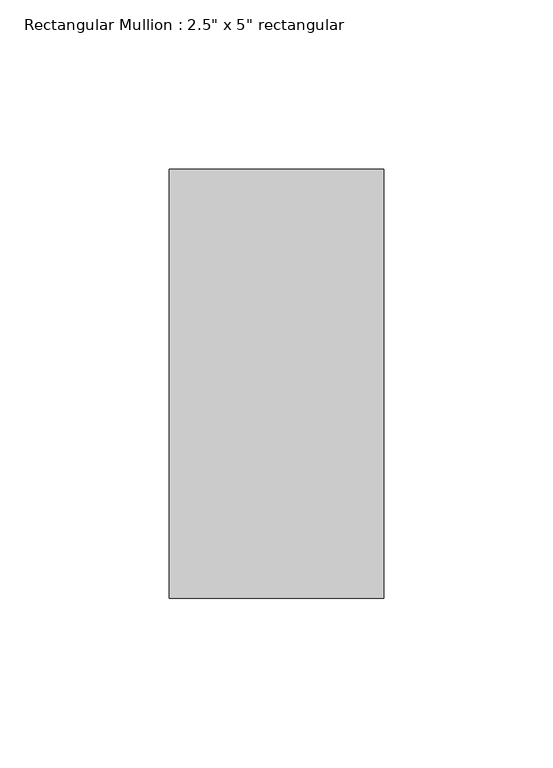
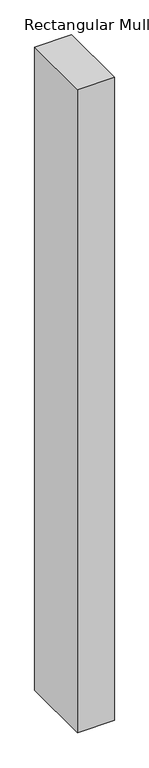
"""IFC4 building model written with IfcOpenShell, lengths in millimetres: member geometry."""

from ifc_helpers import new_model, si_unit, frame, origin, place, context, project, spatial, polyline, outline, extrude, source, transform, mapped, element, save


def member_476d3acb(model_context):
    return source(origin(), model_context, "Body", "SweptSolid", [
        extrude(outline(polyline([(0.0, 63.5), (0.0, -63.5), (-63.5, -63.5), (-63.5, 63.5), (0.0, 63.5)])), frame((0.0, 0.0, -1168.4), z_axis=(0.0, 0.0, 1.0), x_axis=(1.0, 0.0, 0.0)), (0.0, 0.0, 1.0), 1168.4),
    ])


if __name__ == "__main__":
    model = new_model("IFC4")
    model_context = context("Model", 3, world=origin())
    ifc_project = project(units=[si_unit("LENGTHUNIT", "METRE", prefix="MILLI")], contexts=[model_context])
    site = spatial("IfcSite", under=ifc_project)
    building = spatial("IfcBuilding", under=site)
    placement = place(None, origin())
    member_shape = member_476d3acb(model_context)
    element("IfcMember", 1, ObjectType="Rectangular Mullion : 2.5\" x 5\" rectangular", at=placement, inside=building, context=model_context, shape_type="MappedRepresentation", body=[
        mapped(member_shape, transform((0.0, 0.0, 0.0), x_axis=(1.0, 0.0, 0.0), y_axis=(0.0, 1.0, 0.0), z_axis=(0.0, 0.0, 1.0))),
    ])
    save(model, "model.ifc")

# Revit data of these elements
# Type "Rectangular Mullion : 2.5\" x 5\" rectangular"
#   built-in parameter 1007304 = 0.416667 (stored number, unit not read)
#   built-in parameter 1007301 = 0.104167 (stored number, unit not read)
#   built-in parameter 1007300 = 0.104167 (stored number, unit not read)
# Element 1 (IfcMember, "Rectangular Mullion : 2.5\" x 5\" rectangular")
#   Materials on its faces: "Roofing, EPDM Membrane"
# Materials
#   "Roofing, EPDM Membrane": class "Generic", colour RGB 127 127 127, transparency 0, Description = "EPDM roof membrane", Cost = 0
